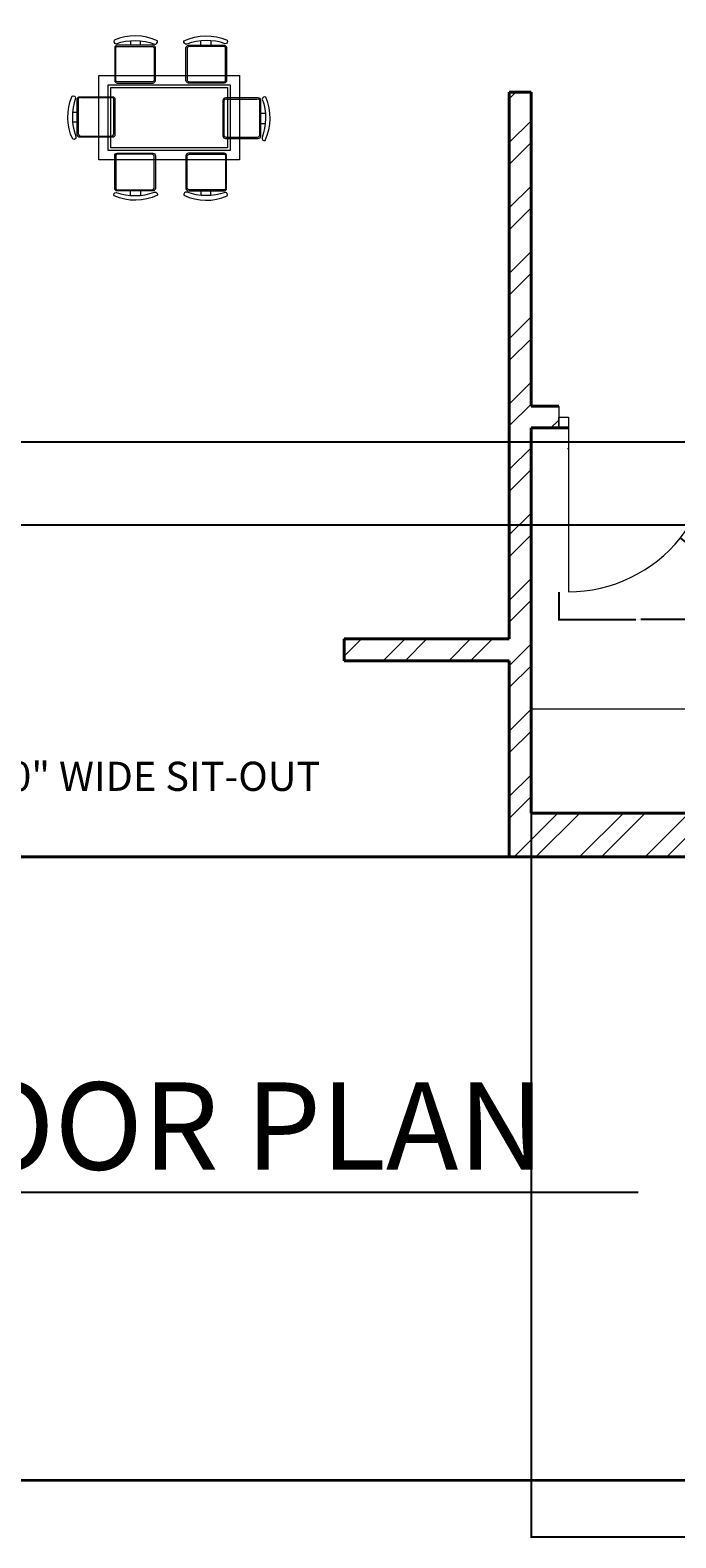
# Model space of a CAD drawing. Units: inches. Extents: x 1355 to 2746, y 1171 to 2751.
# Tile 2 of 24: x 1697 to 1830, y 1171 to 1482. Entities that reach past the tile are written whole.
import ezdxf

# ---------------------------------------------------------------- set-up
doc = ezdxf.new("R2010")
doc.units = ezdxf.units.IN
for name, color, linetype, lineweight in [('A-ANNO-DIMS', 2, 'Continuous', 18), ('A-ANNO-TITL', 7, 'Continuous', 25), ('A-ANNO-TTLB', 7, 'Continuous', 35), ('A-AREA-IDEN', 7, 'Continuous', 18), ('A-DOOR', 3, 'Continuous', 20), ('A-FLOR-CASE', 30, 'Continuous', 20), ('A-FURN', 8, 'Continuous', 13), ('A-WALL', 7, 'Continuous', 40), ('A-WALL-PATT', 252, 'Continuous', 13)]:
    doc.layers.add(name, color=color, linetype=linetype, lineweight=lineweight)
doc.styles.get("Standard").update_dxf_attribs({"font": 'arial.ttf'})
doc.dimstyles.get("Standard").update_dxf_attribs({"dimtxt": 0.18, "dimasz": 0.18, "dimexe": 0.18, "dimexo": 0.0625, "dimgap": 0.09, "dimtad": 0, "dimtih": 1, "dimtoh": 1, "dimdec": 4, "dimzin": 0, "dimdsep": 46, "dimtxsty": 'Standard', "dimcen": 0.09, "dimadec": 0, "dimazin": 0, "dimtfac": 1, "dimtdec": 4, "dimtofl": 0, "dimtmove": 0, "dimatfit": 3, "dimfxl": 1, "dimtolj": 1, "dimtzin": 0, "dimarcsym": 0})

# ---------------------------------------------------------------- blocks, each defined once
blk = doc.blocks.new('TABLE-DINING')
for points in [[(0, 17.41), (29.01, 17.41), (29.01, 0), (0, 0)], [(1.93, 15.47), (27.08, 15.47), (27.08, 1.93), (1.93, 1.93)], [(2.51, 14.89), (26.5, 14.89), (26.5, 2.51), (2.51, 2.51)]]:
    blk.add_lwpolyline(points, close=True)
blk = doc.blocks.new('DOOR-KITCHEN-S')
for p, q in [((0, 38.25), (0, 33.75)), ((32.75, 38.25), (32.75, 33.89)), ((0, 33.75), (0, 36)), ((0, 36), (2, 36)), ((2, 36), (2, 0)), ((32.75, 36), (30.75, 36)), ((32.75, 33.89), (32.75, 36))]:
    blk.add_line(p, q)
blk.add_arc((2, 29.48), 29.48, 270, 12.7851)
blk = doc.blocks.new('*D74')
at = {"layer": 'A-ANNO-DIMS', "color": 0, "lineweight": -2, "transparency": 16777216}
for p, q in [((1805.41, 1365.85), (1805.41, 1360)), ((1838.15, 1365.85), (1838.15, 1360)), ((1805.59, 1360.18), (1821.25, 1360.18)), ((1837.97, 1360.18), (1822.31, 1360.18))]:
    blk.add_line(p, q, dxfattribs=at)
at = {"layer": 'A-ANNO-DIMS', "color": 0, "transparency": 16777216}
for points in [[(1805.59, 1360.21), (1805.59, 1360.15), (1805.41, 1360.18)], [(1837.97, 1360.21), (1837.97, 1360.15), (1838.15, 1360.18)]]:
    blk.add_solid(points, dxfattribs=at)
at = {"layer": 'Defpoints', "color": 0, "transparency": 16777216}
for p in [(1805.41, 1365.92), (1838.15, 1365.92), (1838.15, 1360.18)]:
    blk.add_point(p, dxfattribs=at)
at = {"layer": 'A-ANNO-DIMS', "color": 0, "transparency": 16777216, "insert": (1821.78, 1360.18), "char_height": 0.18, "attachment_point": 5}
blk.add_mtext('\\A1;33 TYP.', dxfattribs=at)
blk = doc.blocks.new('*D106')
at = {"layer": 'A-ANNO-DIMS', "color": 0, "lineweight": -2, "transparency": 16777216}
for p, q in [((2031.09, 1557.85), (1407.53, 1557.85)), ((1407.71, 1557.67), (1407.71, 1434.76)), ((1407.71, 1311.48), (1407.71, 1434.39)), ((2080.33, 1311.3), (1407.53, 1311.3))]:
    blk.add_line(p, q, dxfattribs=at)
at = {"layer": 'A-ANNO-DIMS', "color": 0, "transparency": 16777216}
for points in [[(1407.68, 1557.67), (1407.74, 1557.67), (1407.71, 1557.85)], [(1407.68, 1311.48), (1407.74, 1311.48), (1407.71, 1311.3)]]:
    blk.add_solid(points, dxfattribs=at)
at = {"layer": 'Defpoints', "color": 0, "transparency": 16777216}
for p in [(1407.71, 1557.85), (2031.15, 1557.85), (2080.39, 1311.3)]:
    blk.add_point(p, dxfattribs=at)
at = {"layer": 'A-ANNO-DIMS', "color": 0, "transparency": 16777216, "insert": (1407.71, 1434.57), "char_height": 0.18, "attachment_point": 5}
blk.add_mtext('\\A1;246.54', dxfattribs=at)
blk = doc.blocks.new('*D141')
at = {"layer": 'A-ANNO-DIMS', "color": 0, "lineweight": -2, "transparency": 16777216}
for p, q in [((1799.71, 1320.24), (1799.71, 1171.06)), ((1931.71, 1320.24), (1931.71, 1171.06)), ((1799.89, 1171.24), (1865.43, 1171.24)), ((1931.53, 1171.24), (1865.99, 1171.24))]:
    blk.add_line(p, q, dxfattribs=at)
at = {"layer": 'A-ANNO-DIMS', "color": 0, "transparency": 16777216}
for points in [[(1799.89, 1171.27), (1799.89, 1171.21), (1799.71, 1171.24)], [(1931.53, 1171.27), (1931.53, 1171.21), (1931.71, 1171.24)]]:
    blk.add_solid(points, dxfattribs=at)
at = {"layer": 'Defpoints', "color": 0, "transparency": 16777216}
for p in [(1799.71, 1320.3), (1931.71, 1320.3), (1931.71, 1171.24)]:
    blk.add_point(p, dxfattribs=at)
at = {"layer": 'A-ANNO-DIMS', "color": 0, "transparency": 16777216, "insert": (1865.71, 1171.24), "char_height": 0.18, "attachment_point": 5}
blk.add_mtext('\\A1;132', dxfattribs=at)
blk = doc.blocks.new('*D147')
at = {"layer": 'A-ANNO-DIMS', "color": 0, "lineweight": -2, "transparency": 16777216}
for p, q in [((1913.47, 1396.75), (1407.53, 1396.75)), ((1407.71, 1396.57), (1407.71, 1388.37)), ((1407.71, 1379.8), (1407.71, 1388.01)), ((1913.47, 1379.62), (1407.53, 1379.62))]:
    blk.add_line(p, q, dxfattribs=at)
at = {"layer": 'A-ANNO-DIMS', "color": 0, "transparency": 16777216}
for points in [[(1407.68, 1396.57), (1407.74, 1396.57), (1407.71, 1396.75)], [(1407.68, 1379.8), (1407.74, 1379.8), (1407.71, 1379.62)]]:
    blk.add_solid(points, dxfattribs=at)
at = {"layer": 'Defpoints', "color": 0, "transparency": 16777216}
for p in [(1407.71, 1396.75), (1913.53, 1396.75), (1913.53, 1379.62)]:
    blk.add_point(p, dxfattribs=at)
at = {"layer": 'A-ANNO-DIMS', "color": 0, "transparency": 16777216, "insert": (1407.71, 1388.19), "char_height": 0.18, "attachment_point": 5}
blk.add_mtext('\\A1;17.13', dxfattribs=at)
blk = doc.blocks.new('*D151')
at = {"layer": 'A-ANNO-DIMS', "color": 0, "lineweight": -2, "transparency": 16777216}
for p, q in [((1807.32, 1395.39), (1807.5, 1395.39)), ((1807.41, 1395.3), (1807.41, 1395.48)), ((1844.26, 1365.96), (1830.58, 1376.89)), ((1844.44, 1365.96), (1844.26, 1365.96))]:
    blk.add_line(p, q, dxfattribs=at)
at = {"layer": 'A-ANNO-DIMS', "color": 0, "transparency": 16777216}
blk.add_solid([(1830.6, 1376.91), (1830.56, 1376.86), (1830.44, 1377)], dxfattribs=at)
at = {"layer": 'Defpoints', "color": 0, "transparency": 16777216}
for p in [(1807.41, 1395.39), (1830.44, 1377)]:
    blk.add_point(p, dxfattribs=at)
at = {"layer": 'A-ANNO-DIMS', "color": 0, "transparency": 16777216, "insert": (1844.99, 1365.96), "char_height": 0.18, "attachment_point": 5}
blk.add_mtext('\\A1;R29.477', dxfattribs=at)

msp = doc.modelspace()

# ---------------------------------------------------------------- hatches: boundary and pattern name
at = {"layer": 'A-WALL-PATT'}
h = msp.add_hatch(dxfattribs=at)
h.set_pattern_fill('ANSI32', color=256)
h.paths.add_polyline_path([(1660.2083, 2139.3018), (1614.5977, 2139.3018), (1614.5977, 2130.3018), (1655.7083, 2130.3018), (1655.7083, 1981.8018), (1660.2083, 1981.8018), (1660.2083, 2090.7225), (1692.5832, 2090.7225), (1692.5832, 2095.2225), (1660.2083, 2095.2225)])
h.paths.add_polyline_path([(1523.7083, 2130.3018), (1554.5977, 2130.3018), (1554.5977, 2134.8018), (1554.5977, 2139.3018), (1514.7083, 2139.3018), (1514.7083, 2071.8385), (1523.7083, 2071.8385)])
h.paths.add_polyline_path([(1940.7083, 2139.3018), (1883.7928, 2139.3018), (1883.7928, 2130.3018), (1931.7083, 2130.3018), (1931.7083, 2098.3333), (1940.7083, 2098.3333)])
h.paths.add_polyline_path([(1799.7083, 2130.3018), (1823.7928, 2130.3018), (1823.7928, 2134.8018), (1823.7928, 2139.3018), (1795.2083, 2139.3018), (1795.2083, 2130.3018), (1795.2083, 2095.2225), (1759.2134, 2095.2225), (1759.2134, 2090.7225), (1795.2083, 2090.7225), (1795.2083, 1981.8018), (1799.7083, 1981.8018), (1799.7083, 1986.3018)])
h.paths.add_polyline_path([(1940.7083, 2038.3333), (1931.7083, 2038.3333), (1931.7083, 1986.3018), (1832.7083, 1986.3018), (1832.7083, 1947.1338), (1837.2083, 1947.1338), (1837.2083, 1981.8018), (1931.7083, 1981.8018), (1931.7083, 1967.1939), (1940.7083, 1967.1939)])
h.paths.add_polyline_path([(1940.7083, 1943.1939), (1931.7083, 1943.1939), (1931.7083, 1921.8018), (1837.2083, 1921.8018), (1837.2083, 1926.0511), (1832.7083, 1926.0511), (1832.7083, 1917.3018), (1931.7083, 1917.3018), (1931.7083, 1908.3321), (1940.7083, 1908.3321)])
h.paths.add_polyline_path([(1940.7083, 1884.3321), (1931.7083, 1884.3321), (1931.7083, 1869.3018), (1899.4583, 1869.3018), (1899.4583, 1864.8018), (1931.7083, 1864.8018), (1931.7083, 1773.3018), (1786.5143, 1773.3018), (1786.5143, 1764.3018), (1844.7083, 1764.3018), (1844.7083, 1748.9343), (1853.7083, 1748.9343), (1853.7083, 1764.3018), (1931.7083, 1764.3018), (1931.7083, 1652.9424), (1940.7083, 1652.9424)])
h.paths.add_polyline_path([(1799.7083, 1864.8018), (1806.0522, 1864.8018), (1806.0522, 1867.0518), (1806.0522, 1869.3018), (1799.7083, 1869.3018), (1799.7083, 1917.3018), (1799.7083, 1921.8018), (1795.2083, 1921.8018), (1795.2083, 1773.3018), (1799.7083, 1773.3018)])
h.paths.add_polyline_path([(1872.8988, 1867.0518), (1872.8988, 1869.3018), (1867.2083, 1869.3018), (1867.2083, 1917.3018), (1862.7083, 1917.3018), (1862.7083, 1869.3018), (1836.9546, 1869.3018), (1836.9546, 1864.8018), (1862.7083, 1864.8018), (1872.8988, 1864.8018)])
h.paths.add_polyline_path([(1749.2197, 1773.3018), (1655.7083, 1773.3018), (1523.7083, 1773.3018), (1523.7083, 1828.4963), (1514.7083, 1828.4963), (1514.7083, 1753.9033), (1519.2083, 1753.9033), (1523.7083, 1753.9033), (1523.7083, 1764.3018), (1655.7083, 1764.3018), (1749.2197, 1764.3018), (1749.2197, 1768.8018)])
h.paths.add_polyline_path([(1660.2083, 1921.8018), (1655.7083, 1921.8018), (1655.7083, 1917.3018), (1655.7083, 1773.3018), (1660.2083, 1773.3018)])
h.paths.add_polyline_path([(1523.7083, 2011.8385), (1514.7083, 2011.8385), (1514.7083, 1973.114), (1519.2083, 1973.114), (1523.7083, 1973.114), (1523.7083, 1976.8227), (1523.7083, 1981.8018), (1618.2083, 1981.8018), (1618.2083, 1921.8018), (1553.707, 1921.8018), (1553.707, 1917.3018), (1622.7083, 1917.3018), (1622.7083, 1919.5518), (1622.7083, 1921.8018), (1622.7083, 1986.3018), (1523.7083, 1986.3018)])
h.paths.add_polyline_path([(1529.6686, 1919.5518), (1529.6686, 1921.8018), (1523.7083, 1921.8018), (1523.7083, 1949.114), (1514.7083, 1949.114), (1514.7083, 1888.4963), (1523.7083, 1888.4963), (1523.7083, 1917.3018), (1529.6686, 1917.3018)])
h.paths.add_polyline_path([(1538.9419, 1775.643), (1585.5504, 1775.643), (1585.5504, 1798.0318), (1538.9419, 1798.0318)], flags=25)
h.paths.add_polyline_path([(1696.7097, 1497.3356), (1769.5651, 1497.3356), (1769.5651, 1523.4559), (1696.7097, 1523.4559)], flags=9)
h.paths.add_polyline_path([(1629.1643, 1230.5133), (1877.0879, 1230.5133), (1877.0879, 1267.606), (1629.1643, 1267.606)], flags=9)
h.paths.add_polyline_path([(2533.4462, 2215.4033), (2579.9292, 2215.4033), (2579.9292, 2231.889), (2533.4462, 2231.889)], flags=9)
h.paths.add_polyline_path([(2540.822, 2515.6945), (2594.2245, 2515.6945), (2594.2245, 2545.5463), (2540.822, 2545.5463)], flags=9)
h.paths.add_polyline_path([(2535.9857, 2588.2819), (2582.4687, 2588.2819), (2582.4687, 2604.7675), (2535.9857, 2604.7675)], flags=9)
h.paths.add_polyline_path([(2537.1627, 2617.1172), (2649.1245, 2617.1172), (2649.1245, 2633.6029), (2537.1627, 2633.6029)], flags=9)
h.paths.add_polyline_path([(2218.0051, 2168.228), (2363.9573, 2168.228), (2363.9573, 2205.3208), (2218.0051, 2205.3208)], flags=9)
h.paths.add_polyline_path([(1650.2156, 2165.3631), (1800.3547, 2165.3631), (1800.3547, 2202.4559), (1650.2156, 2202.4559)], flags=9)
h.paths.add_polyline_path([(2553.9592, 1610.7663), (2588.4203, 1610.7663), (2588.4203, 1660.2233), (2553.9592, 1660.2233)], flags=9)
h.paths.add_polyline_path([(1549.0868, 1648.2033), (1595.6952, 1648.2033), (1595.6952, 1670.5921), (1549.0868, 1670.5921)], flags=9)
h.paths.add_polyline_path([(1546.9525, 1502.0931), (1583.3413, 1502.0931), (1583.3413, 1524.4819), (1546.9525, 1524.4819)], flags=9)
h.paths.add_polyline_path([(1540.7704, 1433.4431), (1587.3788, 1433.4431), (1587.3788, 1455.8319), (1540.7704, 1455.8319)], flags=9)
h.paths.add_polyline_path([(1683.6524, 1321.5269), (1760.6169, 1321.5269), (1760.6169, 1333.8911), (1683.6524, 1333.8911)], flags=9)
h.paths.add_polyline_path([(1832.0485, 1356.0874), (1873.0989, 1356.0874), (1873.0989, 1378.4762), (1832.0485, 1378.4762)], flags=9)
h.paths.add_polyline_path([(1877.9694, 1431.2138), (1926.3827, 1431.2138), (1926.3827, 1453.578), (1877.9694, 1453.578)], flags=9)
h.paths.add_polyline_path([(1847.3106, 1499.8371), (1883.6994, 1499.8371), (1883.6994, 1522.2259), (1847.3106, 1522.2259)], flags=9)
h.paths.add_polyline_path([(1813.7015, 1640.7287), (1860.3099, 1640.7287), (1860.3099, 1663.1175), (1813.7015, 1663.1175)], flags=9)
h.paths.add_polyline_path([(1876.2576, 1710.2471), (1912.9452, 1710.2471), (1912.9452, 1732.6359), (1876.2576, 1732.6359)], flags=25)
h.paths.add_polyline_path([(1695.9163, 1715.3064), (1736.9668, 1715.3064), (1736.9668, 1737.6952), (1695.9163, 1737.6952)], flags=9)
h.paths.add_polyline_path([(1881.8583, 1888.9094), (1930.2717, 1888.9094), (1930.2717, 1911.2737), (1881.8583, 1911.2737)], flags=9)
h.paths.add_polyline_path([(1823.9298, 1798.6431), (1864.9803, 1798.6431), (1864.9803, 1821.0319), (1823.9298, 1821.0319)], flags=25)
h.paths.add_polyline_path([(1845.6062, 1948.1408), (1881.995, 1948.1408), (1881.995, 1970.5296), (1845.6062, 1970.5296)], flags=25)
h.paths.add_polyline_path([(1849.027, 1991.5151), (1895.6355, 1991.5151), (1895.6355, 2013.9039), (1849.027, 2013.9039)], flags=25)
h.paths.add_polyline_path([(1684.9725, 2113.8416), (1764.2658, 2113.8416), (1764.2658, 2126.2058), (1684.9725, 2126.2058)], flags=9)
h.paths.add_polyline_path([(1688.6193, 1913.0676), (1776.2005, 1913.0676), (1776.2005, 1935.4564), (1688.6193, 1935.4564)], flags=9)
h.paths.add_polyline_path([(1571.4689, 1930.9816), (1607.8577, 1930.9816), (1607.8577, 1953.3704), (1571.4689, 1953.3704)], flags=25)
h.paths.add_polyline_path([(1535.3581, 1998.3125), (1581.9665, 1998.3125), (1581.9665, 2020.7014), (1535.3581, 2020.7014)], flags=9)
h = msp.add_hatch(dxfattribs=at)
h.set_pattern_fill('ANSI32', color=256)
h.paths.add_polyline_path([(1749.2197, 1686.3018), (1732.6892, 1686.3018), (1523.7083, 1686.3018), (1523.7083, 1705.9033), (1514.7083, 1705.9033), (1514.7083, 1647.8732), (1519.2083, 1647.8732), (1523.7083, 1647.8732), (1523.7083, 1677.3018), (1655.7083, 1677.3018), (1655.7083, 1528.8018), (1660.2083, 1528.8018), (1660.2083, 1677.3018), (1732.6892, 1677.3018), (1749.2197, 1677.3018)])
h.paths.add_polyline_path([(1931.7083, 1686.3018), (1853.7083, 1686.3018), (1853.7083, 1703.5696), (1844.7083, 1703.5696), (1844.7083, 1686.3018), (1788.0274, 1686.3018), (1788.0274, 1677.3018), (1795.2083, 1677.3018), (1795.2083, 1528.8018), (1799.7083, 1528.8018), (1799.7083, 1677.3018), (1844.7083, 1677.3018), (1931.7083, 1677.3018)])
h.paths.add_polyline_path([(1931.7083, 1533.3018), (1844.7083, 1533.3018), (1832.7083, 1533.3018), (1832.7083, 1531.0518), (1832.7083, 1528.8018), (1832.7083, 1495.7519), (1837.2083, 1495.7519), (1837.2083, 1528.8018), (1931.7083, 1528.8018)])
h.paths.add_polyline_path([(1940.7083, 1592.9424), (1931.7083, 1592.9424), (1931.7083, 1506.7845), (1940.7083, 1506.7845)])
h.paths.add_polyline_path([(1940.7083, 1482.7845), (1936.2083, 1482.7845), (1931.7083, 1482.7845), (1931.7083, 1320.3018), (1880.7083, 1320.3018), (1880.7083, 1311.3018), (1940.7083, 1311.3018)])
h.paths.add_polyline_path([(1931.7083, 1468.8018), (1844.7083, 1468.8018), (1837.2083, 1468.8018), (1837.2083, 1474.34), (1832.7083, 1474.34), (1832.7083, 1468.8018), (1832.7083, 1464.3018), (1844.7083, 1464.3018), (1931.7083, 1464.3018)])
h.paths.add_polyline_path([(1863.8571, 1464.3018), (1859.3571, 1464.3018), (1859.3571, 1404.1662), (1838.1542, 1404.1662), (1838.1542, 1399.8018), (1869.4185, 1399.8018), (1869.4185, 1402.0518), (1869.4185, 1404.3018), (1863.8571, 1404.3018)])
h.paths.add_polyline_path([(1799.7083, 1399.6662), (1805.4082, 1399.6662), (1805.4082, 1401.9162), (1805.4082, 1404.1662), (1799.7083, 1404.1662), (1799.7083, 1464.3018), (1799.7083, 1468.8018), (1795.2083, 1468.8018), (1795.2083, 1356.2098), (1761.2597, 1356.2098), (1761.2597, 1351.7098), (1795.2083, 1351.7098), (1795.2083, 1320.3018), (1795.2083, 1311.3018), (1844.7083, 1311.3018), (1844.7083, 1315.8018), (1844.7083, 1320.3018), (1799.7083, 1320.3018)])
h.paths.add_polyline_path([(1692.9218, 1356.2098), (1660.2083, 1356.2098), (1660.2083, 1430.786), (1657.9583, 1430.786), (1655.7083, 1430.786), (1655.7083, 1320.3018), (1611.934, 1320.3018), (1611.934, 1311.3018), (1660.2083, 1311.3018), (1660.2083, 1351.7098), (1692.9218, 1351.7098)])
h.paths.add_polyline_path([(1523.7083, 1372.653), (1514.7083, 1372.653), (1514.7083, 1311.3018), (1551.934, 1311.3018), (1551.934, 1315.8018), (1551.934, 1320.3018), (1523.7083, 1320.3018)])
h.paths.add_polyline_path([(1523.7083, 1490.9023), (1514.7083, 1490.9023), (1514.7083, 1432.653), (1519.2083, 1432.653), (1523.7083, 1432.653)])
h.paths.add_polyline_path([(1660.2083, 1468.8018), (1622.7083, 1468.8018), (1622.7083, 1473.1566), (1618.2083, 1473.1566), (1618.2083, 1468.8018), (1523.7083, 1468.8018), (1523.7083, 1464.3018), (1655.7083, 1464.3018), (1655.7083, 1460.5634), (1660.2083, 1460.5634)])
h.paths.add_polyline_path([(1523.7083, 1587.8732), (1514.7083, 1587.8732), (1514.7083, 1514.9023), (1519.2083, 1514.9023), (1523.7083, 1514.9023)])
h.paths.add_polyline_path([(1622.7083, 1533.3018), (1523.7083, 1533.3018), (1523.7083, 1528.8018), (1618.2083, 1528.8018), (1618.2083, 1494.4205), (1622.7083, 1494.4205), (1622.7083, 1528.8018)])
h.paths.add_polyline_path([(1696.7097, 1497.3356), (1769.5651, 1497.3356), (1769.5651, 1523.4559), (1696.7097, 1523.4559)], flags=9)
h.paths.add_polyline_path([(1629.1643, 1230.5133), (1877.0879, 1230.5133), (1877.0879, 1267.606), (1629.1643, 1267.606)], flags=9)
h.paths.add_polyline_path([(2533.4462, 2215.4033), (2579.9292, 2215.4033), (2579.9292, 2231.889), (2533.4462, 2231.889)], flags=9)
h.paths.add_polyline_path([(2540.822, 2515.6945), (2594.2245, 2515.6945), (2594.2245, 2545.5463), (2540.822, 2545.5463)], flags=9)
h.paths.add_polyline_path([(2535.9857, 2588.2819), (2582.4687, 2588.2819), (2582.4687, 2604.7675), (2535.9857, 2604.7675)], flags=9)
h.paths.add_polyline_path([(2537.1627, 2617.1172), (2649.1245, 2617.1172), (2649.1245, 2633.6029), (2537.1627, 2633.6029)], flags=9)
h.paths.add_polyline_path([(2218.0051, 2168.228), (2363.9573, 2168.228), (2363.9573, 2205.3208), (2218.0051, 2205.3208)], flags=9)
h.paths.add_polyline_path([(1650.2156, 2165.3631), (1800.3547, 2165.3631), (1800.3547, 2202.4559), (1650.2156, 2202.4559)], flags=9)
h.paths.add_polyline_path([(2553.9592, 1610.7663), (2588.4203, 1610.7663), (2588.4203, 1660.2233), (2553.9592, 1660.2233)], flags=9)
h.paths.add_polyline_path([(1549.0868, 1648.2033), (1595.6952, 1648.2033), (1595.6952, 1670.5921), (1549.0868, 1670.5921)], flags=25)
h.paths.add_polyline_path([(1546.9525, 1502.0931), (1583.3413, 1502.0931), (1583.3413, 1524.4819), (1546.9525, 1524.4819)], flags=25)
h.paths.add_polyline_path([(1540.7704, 1433.4431), (1587.3788, 1433.4431), (1587.3788, 1455.8319), (1540.7704, 1455.8319)], flags=9)
h.paths.add_polyline_path([(1683.6524, 1321.5269), (1760.6169, 1321.5269), (1760.6169, 1333.8911), (1683.6524, 1333.8911)], flags=9)
h.paths.add_polyline_path([(1832.0485, 1356.0874), (1873.0989, 1356.0874), (1873.0989, 1378.4762), (1832.0485, 1378.4762)], flags=9)
h.paths.add_polyline_path([(1877.9694, 1431.2138), (1926.3827, 1431.2138), (1926.3827, 1453.578), (1877.9694, 1453.578)], flags=9)
h.paths.add_polyline_path([(1847.3106, 1499.8371), (1883.6994, 1499.8371), (1883.6994, 1522.2259), (1847.3106, 1522.2259)], flags=25)
h.paths.add_polyline_path([(1813.7015, 1640.7287), (1860.3099, 1640.7287), (1860.3099, 1663.1175), (1813.7015, 1663.1175)], flags=25)
h.paths.add_polyline_path([(1876.2576, 1710.2471), (1912.9452, 1710.2471), (1912.9452, 1732.6359), (1876.2576, 1732.6359)], flags=9)
h.paths.add_polyline_path([(1695.9163, 1715.3064), (1736.9668, 1715.3064), (1736.9668, 1737.6952), (1695.9163, 1737.6952)], flags=9)
h.paths.add_polyline_path([(1881.8583, 1888.9094), (1930.2717, 1888.9094), (1930.2717, 1911.2737), (1881.8583, 1911.2737)], flags=9)
h.paths.add_polyline_path([(1823.9298, 1798.6431), (1864.9803, 1798.6431), (1864.9803, 1821.0319), (1823.9298, 1821.0319)], flags=9)
h.paths.add_polyline_path([(1845.6062, 1948.1408), (1881.995, 1948.1408), (1881.995, 1970.5296), (1845.6062, 1970.5296)], flags=9)
h.paths.add_polyline_path([(1849.027, 1991.5151), (1895.6355, 1991.5151), (1895.6355, 2013.9039), (1849.027, 2013.9039)], flags=9)
h.paths.add_polyline_path([(1684.9725, 2113.8416), (1764.2658, 2113.8416), (1764.2658, 2126.2058), (1684.9725, 2126.2058)], flags=9)
h.paths.add_polyline_path([(1688.6193, 1913.0676), (1776.2005, 1913.0676), (1776.2005, 1935.4564), (1688.6193, 1935.4564)], flags=9)
h.paths.add_polyline_path([(1538.9419, 1775.643), (1585.5504, 1775.643), (1585.5504, 1798.0318), (1538.9419, 1798.0318)], flags=9)
h.paths.add_polyline_path([(1571.4689, 1930.9816), (1607.8577, 1930.9816), (1607.8577, 1953.3704), (1571.4689, 1953.3704)], flags=9)
h.paths.add_polyline_path([(1535.3581, 1998.3125), (1581.9665, 1998.3125), (1581.9665, 2020.7014), (1535.3581, 2020.7014)], flags=9)

# ---------------------------------------------------------------- linework, layer by layer
at = {"layer": 'A-ANNO-TITL'}
msp.add_line((1583.8987, 1242.2388), (1821.7611, 1242.2388), dxfattribs=at)
at = {"layer": 'A-ANNO-TTLB'}
msp.add_lwpolyline([(1355.0901, 2751.4741), (2746.1804, 2751.4741), (2746.1804, 1182.883), (1355.0901, 1182.883)], close=True, dxfattribs=at)
at = {"layer": 'A-FLOR-CASE'}
msp.add_line((1799.7083, 1341.7851), (1910.8841, 1341.7851), dxfattribs=at)
at = {"layer": 'A-FURN'}
for points in [[(1714.3247, 1478.7913, -0.17580919), (1722.2264, 1478.7315, 0.57839206), (1722.825, 1479.3897, 0.21452438), (1713.9057, 1479.5094, 0.55201397), (1714.3247, 1478.7913, -0.06507904)], [(1721.8912, 1478.4742), (1714.5555, 1478.4742, 0.41421356), (1714.0423, 1477.961), (1714.0423, 1471.216, 0.41421356), (1714.5555, 1470.7028), (1721.8912, 1470.7028, 0.41421356), (1722.4044, 1471.216), (1722.4044, 1477.961, 0.41421356), (1721.8912, 1478.4742)], [(1719.3145, 1478.4742), (1719.3145, 1479.4019, -0.06475861)], [(1728.8786, 1478.7315, -0.57839206), (1728.28, 1479.3897, -0.21452438), (1737.1993, 1479.5094, -0.55201397), (1736.7803, 1478.7913, 0.1758092), (1728.8786, 1478.7315)], [(1736.5495, 1478.4742, -0.41421356), (1737.0627, 1477.961), (1737.0627, 1471.216, -0.41421356), (1736.5495, 1470.7028), (1729.2138, 1470.7028, -0.41421356), (1728.7006, 1471.216), (1728.7006, 1477.961, -0.41421356), (1729.2138, 1478.4742), (1736.5495, 1478.4742)], [(1731.7905, 1478.4742), (1731.7905, 1479.4019, 0.06475861)], [(1706.058, 1459.7099, -0.57839206), (1705.3998, 1459.1113, -0.21452438), (1705.2801, 1468.0307, -0.55201397), (1705.9982, 1467.6116, 0.17580937), (1706.058, 1459.7099)], [(1706.3153, 1467.3808, -0.41421356), (1706.8285, 1467.8941), (1713.5735, 1467.8941, -0.41421356), (1714.0867, 1467.3808), (1714.0867, 1460.0452, -0.41421356), (1713.5735, 1459.532), (1706.8285, 1459.532, -0.41421356), (1706.3153, 1460.0452), (1706.3153, 1467.3808)], [(1744.0906, 1467.1296, 0.41421356), (1743.5774, 1467.6428), (1736.8324, 1467.6428, 0.41421356), (1736.3191, 1467.1296), (1736.3191, 1459.7939, 0.41421356), (1736.8324, 1459.2807), (1743.5774, 1459.2807, 0.41421356), (1744.0906, 1459.7939), (1744.0906, 1467.1296)], [(1744.4077, 1467.3604, -0.17580919), (1744.3479, 1459.4587, 0.57839206), (1745.0061, 1458.8601, 0.21452438), (1745.1258, 1467.7794, 0.55201397), (1744.4077, 1467.3604, -0.06507904)], [(1706.3153, 1462.6218), (1705.3876, 1462.6218, 0.06475861)], [(1744.0906, 1462.3706), (1745.0183, 1462.3706, -0.06475861)], [(1721.8912, 1448.491), (1714.5555, 1448.491, -0.41421356), (1714.0423, 1449.0042), (1714.0423, 1455.7492, -0.41421356), (1714.5555, 1456.2624), (1721.8912, 1456.2624, -0.41421356), (1722.4044, 1455.7492), (1722.4044, 1449.0042, -0.41421356), (1721.8912, 1448.491)], [(1736.5495, 1448.491, 0.41421356), (1737.0627, 1449.0042), (1737.0627, 1455.7492, 0.41421356), (1736.5495, 1456.2624), (1729.2138, 1456.2624, 0.41421356), (1728.7006, 1455.7492), (1728.7006, 1449.0042, 0.41421356), (1729.2138, 1448.491), (1736.5495, 1448.491)], [(1722.2264, 1448.2337, -0.57839206), (1722.825, 1447.5755, -0.21452438), (1713.9057, 1447.4558, -0.55201397), (1714.3247, 1448.1739, 0.17580929), (1722.2264, 1448.2337)], [(1719.3145, 1448.491), (1719.3145, 1447.5633, 0.06475861)], [(1736.7803, 1448.1739, -0.17580928), (1728.8786, 1448.2337, 0.57839206), (1728.28, 1447.5755, 0.21452438), (1737.1993, 1447.4558, 0.55201397), (1736.7803, 1448.1739, -0.06507904)], [(1731.7905, 1448.491), (1731.7905, 1447.5633, -0.06475861)]]:
    msp.add_lwpolyline(points, format="xyb", dxfattribs=at)
for points in [[(1714.5586, 1478.243), (1721.6599, 1478.243, -0.41421356), (1722.1732, 1477.7298), (1722.1732, 1471.4472, -0.41421356), (1721.6599, 1470.934), (1714.5586, 1470.934, -0.51206948), (1714.2735, 1471.4472), (1714.2735, 1477.7298, -0.51206948)], [(1736.5464, 1478.243), (1729.445, 1478.243, 0.41421356), (1728.9318, 1477.7298), (1728.9318, 1471.4472, 0.41421356), (1729.445, 1470.934), (1736.5464, 1470.934, 0.51206948), (1736.8315, 1471.4472), (1736.8315, 1477.7298, 0.51206948)], [(1706.5465, 1467.3777), (1706.5465, 1460.2764, 0.41421356), (1707.0597, 1459.7632), (1713.3423, 1459.7632, 0.41421356), (1713.8555, 1460.2764), (1713.8555, 1467.3777, 0.51206948), (1713.3423, 1467.6628), (1707.0597, 1467.6628, 0.51206948)], [(1743.8594, 1467.1265), (1743.8594, 1460.0251, -0.41421356), (1743.3462, 1459.5119), (1737.0636, 1459.5119, -0.41421356), (1736.5503, 1460.0251), (1736.5503, 1467.1265, -0.51206948), (1737.0636, 1467.4116), (1743.3462, 1467.4116, -0.51206948)], [(1714.5586, 1448.7222), (1721.6599, 1448.7222, 0.41421356), (1722.1732, 1449.2354), (1722.1732, 1455.518, 0.41421356), (1721.6599, 1456.0312), (1714.5586, 1456.0312, 0.51206948), (1714.2735, 1455.518), (1714.2735, 1449.2354, 0.51206948)], [(1736.5464, 1448.7222), (1729.445, 1448.7222, -0.41421356), (1728.9318, 1449.2354), (1728.9318, 1455.518, -0.41421356), (1729.445, 1456.0312), (1736.5464, 1456.0312, -0.51206948), (1736.8315, 1455.518), (1736.8315, 1449.2354, -0.51206948)]]:
    msp.add_lwpolyline(points, format="xyb", close=True, dxfattribs=at)
for points in [[(1717.2611, 1479.4188), (1717.2611, 1478.4742)], [(1733.8439, 1479.4188), (1733.8439, 1478.4742)], [(1705.3707, 1464.6752), (1706.3153, 1464.6752)], [(1745.0352, 1464.424), (1744.0906, 1464.424)], [(1717.2611, 1447.5464), (1717.2611, 1448.491)], [(1733.8439, 1447.5464), (1733.8439, 1448.491)]]:
    msp.add_lwpolyline(points, dxfattribs=at)
at = {"layer": 'A-WALL'}
for p, q in [((1795.2083, 1468.8018), (1795.2083, 1356.2098)), ((1799.7083, 1468.8018), (1795.2083, 1468.8018)), ((1799.7083, 1464.3018), (1799.7083, 1468.8018)), ((1799.7083, 1464.3018), (1799.7083, 1404.1662)), ((1805.4082, 1404.1662), (1799.7083, 1404.1662)), ((1799.7083, 1399.6662), (1807.4082, 1399.6662)), ((1799.7083, 1399.6662), (1799.7083, 1320.3018)), ((1795.2083, 1356.2098), (1761.2597, 1356.2098)), ((1761.2597, 1356.2098), (1761.2597, 1351.7098)), ((1761.2597, 1351.7098), (1795.2083, 1351.7098)), ((1795.2083, 1351.7098), (1795.2083, 1320.3018)), ((1795.2083, 1320.3018), (1795.2083, 1311.3018)), ((1931.7083, 1320.3018), (1799.7083, 1320.3018)), ((1660.2083, 1311.3018), (1795.2083, 1311.3018)), ((1940.7083, 1311.3018), (1795.2083, 1311.3018))]:
    msp.add_line(p, q, dxfattribs=at)

# ---------------------------------------------------------------- block references
at = {"layer": 'A-DOOR'}
msp.add_blockref('DOOR-KITCHEN-S', (1805.408, 1365.916), dxfattribs=at)
at = {"layer": 'A-FURN'}
msp.add_blockref('TABLE-DINING', (1710.7363, 1454.8727), dxfattribs=at)

# ---------------------------------------------------------------- texts
at = {"layer": 'A-ANNO-TITL', "insert": (1585.3462, 1264.8825), "char_height": 18, "attachment_point": 1}
msp.add_mtext_dynamic_manual_height_columns('FIRST FLOOR PLAN ', width=423.704908, gutter_width=12.5, heights=[0], dxfattribs=at)
at = {"layer": 'A-AREA-IDEN', "insert": (1685.5003, 1330.9095), "char_height": 6, "attachment_point": 1}
msp.add_mtext_dynamic_manual_height_columns('5\'0" WIDE SIT-OUT', width=135.198856, gutter_width=12.5, heights=[0], dxfattribs=at)

# ---------------------------------------------------------------- dimensions: what is measured, and where the dimension line sits
at = {"layer": 'A-ANNO-DIMS'}
for base, p1, p2, picture, middle in [((1407.7083, 1557.845), (2080.3909, 1311.3018), (2031.1535, 1557.845), '*D106', (1407.7083, 1434.5734)), ((1407.7083, 1396.7528), (1913.531, 1379.6228), (1913.531, 1396.7528), '*D147', (1407.7083, 1388.1878))]:
    dim = msp.add_linear_dim(base=base, p1=p1, p2=p2, angle=90, dimstyle='Standard', override={"dimdec": 2, "dimlfac": 1, "dimrnd": 0, "dimzin": 0, "dimdsep": 46, "dimlunit": 2}, dxfattribs=at)
    dim.commit()
    dim.dimension.update_dxf_attribs({"geometry": picture, "text_midpoint": middle})
dim = msp.add_radius_dim(center=(1807.4082, 1395.3931), mpoint=(1830.4427, 1377.0002), dimstyle='Standard', override={"dimdec": 3, "dimlfac": 1, "dimrnd": 0, "dimzin": 0, "dimdsep": 46, "dimlunit": 2}, dxfattribs=at)
dim.commit()
dim.dimension.update_dxf_attribs({"geometry": '*D151', "text_midpoint": (1844.9932, 1365.9645), "dimtype": 164})
dim = msp.add_linear_dim(base=(1838.1542, 1360.1787), p1=(1805.4082, 1365.9162), p2=(1838.1542, 1365.9162), text='<> TYP.', dimstyle='Standard', override={"dimdec": 0, "dimlfac": 1, "dimrnd": 0, "dimzin": 0, "dimdsep": 46, "dimlunit": 2}, dxfattribs=at)
dim.commit()
dim.dimension.update_dxf_attribs({"geometry": '*D74', "text_midpoint": (1821.7812, 1360.1787)})
dim = msp.add_linear_dim(base=(1931.7083, 1171.2388), p1=(1799.7083, 1320.3018), p2=(1931.7083, 1320.3018), dimstyle='Standard', override={"dimdec": 0, "dimlfac": 1, "dimrnd": 0, "dimzin": 0, "dimdsep": 46, "dimlunit": 2}, dxfattribs=at)
dim.commit()
dim.dimension.update_dxf_attribs({"geometry": '*D141', "text_midpoint": (1865.7083, 1171.2388)})

doc.saveas('drawing.dxf')
